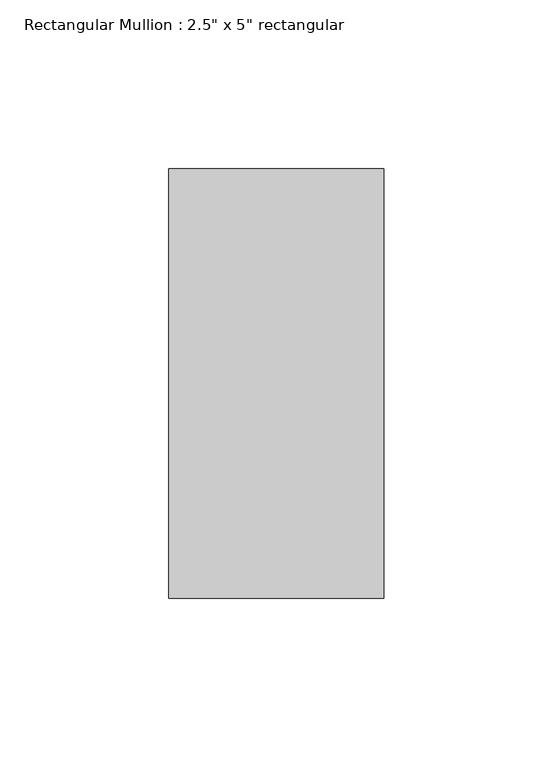
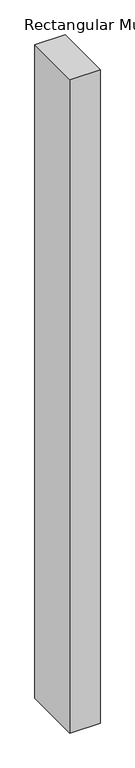
"""IFC4 building model written with IfcOpenShell, lengths in millimetres: member geometry."""

from ifc_helpers import new_model, si_unit, frame, origin, place, context, project, spatial, polyline, outline, extrude, source, transform, mapped, element, save


def member_ee8fd4dd(model_context):
    return source(origin(), model_context, "Body", "SweptSolid", [
        extrude(outline(polyline([(31.75, 63.5), (31.75, -63.5), (-31.75, -63.5), (-31.75, 63.5), (31.75, 63.5)])), frame((0.0, 0.0, -1451.8907014), z_axis=(0.0, 0.0, 1.0), x_axis=(1.0, 0.0, 0.0)), (0.0, 0.0, 1.0), 1451.8907014),
    ])


if __name__ == "__main__":
    model = new_model("IFC4")
    model_context = context("Model", 3, world=origin())
    ifc_project = project(units=[si_unit("LENGTHUNIT", "METRE", prefix="MILLI")], contexts=[model_context])
    site = spatial("IfcSite", under=ifc_project)
    building = spatial("IfcBuilding", under=site)
    placement = place(None, origin())
    member_shape = member_ee8fd4dd(model_context)
    element("IfcMember", 1, ObjectType="Rectangular Mullion : 2.5\" x 5\" rectangular", at=placement, inside=building, context=model_context, shape_type="MappedRepresentation", body=[
        mapped(member_shape, transform((0.0, 0.0, 0.0), x_axis=(1.0, 0.0, 0.0), y_axis=(0.0, 1.0, 0.0), z_axis=(0.0, 0.0, 1.0))),
    ])
    save(model, "model.ifc")

# Revit data of these elements
# Type "Rectangular Mullion : 2.5\" x 5\" rectangular"
#   built-in parameter 1007304 = 0.416667 (stored number, unit not read)
#   built-in parameter 1007301 = 0.104167 (stored number, unit not read)
#   built-in parameter 1007300 = 0.104167 (stored number, unit not read)
# Element 1 (IfcMember, "Rectangular Mullion : 2.5\" x 5\" rectangular")
#   Materials on its faces: "Aluminum"
# Materials
#   "Aluminum": class "Metal", colour RGB 247 247 247, transparency 0, Description = "Aluminum 6061", Cost = 0
